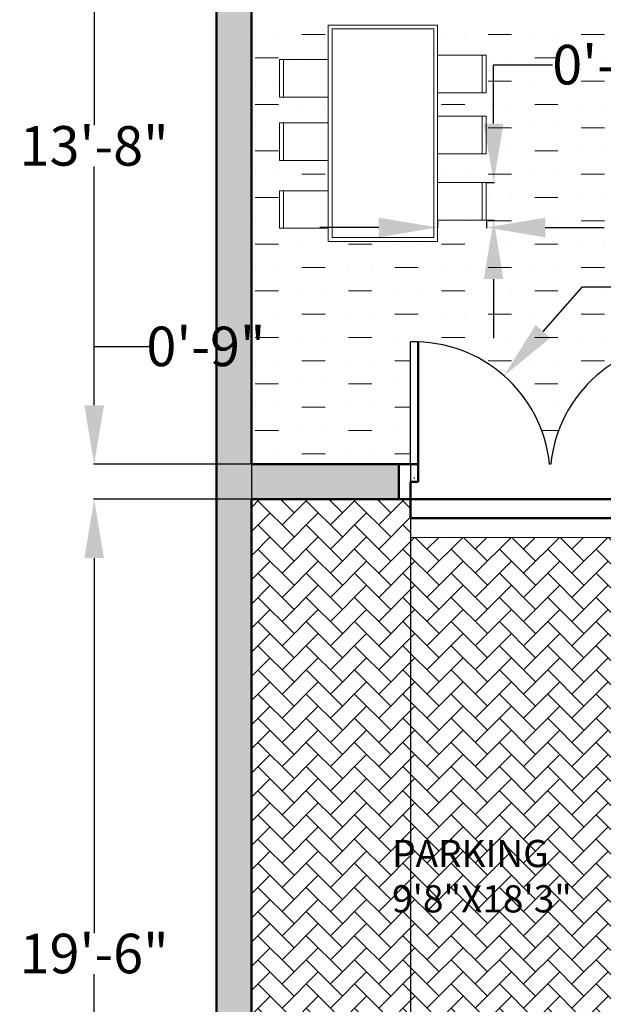
# Model space of a CAD drawing. Units: inches. Extents: x 26 to 14419, y 2 to 3479.
# Tile 2 of 9: x 13608 to 13759, y 2946 to 3199. Entities that reach past the tile are written whole.
import ezdxf

# ---------------------------------------------------------------- set-up
doc = ezdxf.new("R2010")
doc.units = ezdxf.units.IN
doc.header["$MEASUREMENT"] = 0
for name, color, linetype, lineweight in [('A-ANNO-DIMS', 2, 'Continuous', 18), ('A-AREA-IDEN', 7, 'Continuous', 18), ('A-DOOR', 4, 'Continuous', 25), ('A-FLOR-PATT', 252, 'Continuous', 13), ('A-FURN', 8, 'Continuous', 18), ('A-WALL', 7, 'Continuous', 50)]:
    doc.layers.add(name, color=color, linetype=linetype, lineweight=lineweight)
doc.styles.get("Standard").update_dxf_attribs({"font": 'arial.ttf'})
doc.dimstyles.get("Standard").update_dxf_attribs({"dimtxt": 10.18, "dimasz": 15.18, "dimexe": 0.18, "dimexo": 0.0625, "dimgap": 0.09, "dimtad": 0, "dimtih": 1, "dimtoh": 1, "dimdec": 0, "dimzin": 0, "dimdsep": 46, "dimlunit": 3, "dimtxsty": 'Standard', "dimcen": 0.09, "dimadec": 0, "dimazin": 0, "dimtfac": 1, "dimtdec": 0, "dimtofl": 0, "dimtmove": 0, "dimatfit": 3, "dimfxl": 1, "dimtolj": 1, "dimtzin": 0, "dimarcsym": 0})

# ---------------------------------------------------------------- blocks, each defined once
blk = doc.blocks.new('DOOR-DOUBLE')
for p, q in [((0, 0), (0, 31.5)), ((72, 0), (72, 31.5)), ((36.16, 0), (35.84, 0))]:
    blk.add_line(p, q)
for centre, start, end in [((1, -3.5), 5.7368, 91.6366), ((71, -3.5), 88.3634, 174.2632)]:
    blk.add_arc(centre, 35.01, start, end)
blk = doc.blocks.new('CHAIR')
blk.add_line((11.52, 9.68), (11.52, 0))
blk.add_lwpolyline([(0, 9.68), (12.56, 9.68), (12.56, 0), (0, 0)], close=True)
blk = doc.blocks.new('*D23')
at = {"layer": 'A-ANNO-DIMS', "color": 0, "lineweight": -2, "transparency": 16777216}
for p, q in [((13716.08, 3147.8), (13716.08, 3145.8)), ((13728.65, 3147.8), (13728.65, 3145.8)), ((13700.9, 3145.98), (13685.72, 3145.98)), ((13743.83, 3145.98), (13759.01, 3145.98))]:
    blk.add_line(p, q, dxfattribs=at)
at = {"layer": 'A-ANNO-DIMS', "color": 0, "transparency": 16777216}
for points in [[(13700.9, 3148.51), (13700.9, 3143.45), (13716.08, 3145.98)], [(13743.83, 3148.51), (13743.83, 3143.45), (13728.65, 3145.98)]]:
    blk.add_solid(points, dxfattribs=at)
at = {"layer": 'Defpoints', "color": 0, "transparency": 16777216}
for p in [(13716.08, 3147.87), (13728.65, 3147.87), (13728.65, 3145.98)]:
    blk.add_point(p, dxfattribs=at)
at = {"layer": 'A-ANNO-DIMS', "color": 0, "transparency": 16777216, "insert": (13826.02, 3145.98), "char_height": 10.18, "attachment_point": 5}
blk.add_mtext('\\A1;CHAIR 1\'-0 1/2" TYP.', dxfattribs=at)
blk = doc.blocks.new('*D24')
at = {"layer": 'A-ANNO-DIMS', "color": 0, "lineweight": -2, "transparency": 16777216}
for p, q in [((13730.53, 3172.73), (13730.53, 3187.91)), ((13730.53, 3187.91), (13745.71, 3187.91)), ((13728.71, 3157.55), (13730.71, 3157.55)), ((13728.71, 3147.87), (13730.71, 3147.87)), ((13730.53, 3132.69), (13730.53, 3117.51))]:
    blk.add_line(p, q, dxfattribs=at)
at = {"layer": 'A-ANNO-DIMS', "color": 0, "transparency": 16777216}
for points in [[(13728, 3172.73), (13733.06, 3172.73), (13730.53, 3157.55)], [(13728, 3132.69), (13733.06, 3132.69), (13730.53, 3147.87)]]:
    blk.add_solid(points, dxfattribs=at)
at = {"layer": 'Defpoints', "color": 0, "transparency": 16777216}
for p in [(13728.65, 3157.55), (13730.53, 3157.55), (13728.65, 3147.87)]:
    blk.add_point(p, dxfattribs=at)
at = {"layer": 'A-ANNO-DIMS', "color": 0, "transparency": 16777216, "insert": (13788.69, 3187.91), "char_height": 10.18, "attachment_point": 5}
blk.add_mtext('\\A1;0\'-9 1/2" TYP.', dxfattribs=at)
blk = doc.blocks.new('*D56')
at = {"layer": 'A-ANNO-DIMS', "color": 0, "lineweight": -2, "transparency": 16777216}
for p, q in [((13668.03, 3076), (13627.41, 3076)), ((13627.59, 3060.82), (13627.59, 2964.28)), ((13627.59, 2857.18), (13627.59, 2953.71)), ((13668.03, 2842), (13627.41, 2842))]:
    blk.add_line(p, q, dxfattribs=at)
at = {"layer": 'A-ANNO-DIMS', "color": 0, "transparency": 16777216}
for points in [[(13625.06, 3060.82), (13630.12, 3060.82), (13627.59, 3076)], [(13625.06, 2857.18), (13630.12, 2857.18), (13627.59, 2842)]]:
    blk.add_solid(points, dxfattribs=at)
at = {"layer": 'Defpoints', "color": 0, "transparency": 16777216}
for p in [(13627.59, 3076), (13668.09, 3076), (13668.09, 2842)]:
    blk.add_point(p, dxfattribs=at)
at = {"layer": 'A-ANNO-DIMS', "color": 0, "transparency": 16777216, "insert": (13627.59, 2959), "char_height": 10.18, "attachment_point": 5}
blk.add_mtext('\\A1;19\'-6"', dxfattribs=at)
blk = doc.blocks.new('*D57')
at = {"layer": 'A-ANNO-DIMS', "color": 0, "lineweight": -2, "transparency": 16777216}
for p, q in [((13627.59, 3100.18), (13627.59, 3115.36)), ((13627.59, 3115.36), (13642.77, 3115.36)), ((13668.03, 3085), (13627.41, 3085)), ((13668.03, 3076), (13627.41, 3076)), ((13627.59, 3060.82), (13627.59, 3045.64))]:
    blk.add_line(p, q, dxfattribs=at)
at = {"layer": 'A-ANNO-DIMS', "color": 0, "transparency": 16777216}
for points in [[(13625.06, 3100.18), (13630.12, 3100.18), (13627.59, 3085)], [(13625.06, 3060.82), (13630.12, 3060.82), (13627.59, 3076)]]:
    blk.add_solid(points, dxfattribs=at)
at = {"layer": 'Defpoints', "color": 0, "transparency": 16777216}
for p in [(13627.59, 3085), (13668.09, 3085), (13668.09, 3076)]:
    blk.add_point(p, dxfattribs=at)
at = {"layer": 'A-ANNO-DIMS', "color": 0, "transparency": 16777216, "insert": (13656.39, 3115.36), "char_height": 10.18, "attachment_point": 5}
blk.add_mtext('\\A1;0\'-9"', dxfattribs=at)
blk = doc.blocks.new('*D58')
at = {"layer": 'A-ANNO-DIMS', "color": 0, "lineweight": -2, "transparency": 16777216}
for p, q in [((13668.03, 3249), (13627.41, 3249)), ((13627.59, 3233.82), (13627.59, 3172.29)), ((13627.59, 3100.18), (13627.59, 3161.7)), ((13668.03, 3085), (13627.41, 3085))]:
    blk.add_line(p, q, dxfattribs=at)
at = {"layer": 'A-ANNO-DIMS', "color": 0, "transparency": 16777216}
for points in [[(13625.06, 3233.82), (13630.12, 3233.82), (13627.59, 3249)], [(13625.06, 3100.18), (13630.12, 3100.18), (13627.59, 3085)]]:
    blk.add_solid(points, dxfattribs=at)
at = {"layer": 'Defpoints', "color": 0, "transparency": 16777216}
for p in [(13627.59, 3249), (13668.09, 3249), (13668.09, 3085)]:
    blk.add_point(p, dxfattribs=at)
at = {"layer": 'A-ANNO-DIMS', "color": 0, "transparency": 16777216, "insert": (13627.59, 3167), "char_height": 10.18, "attachment_point": 5}
blk.add_mtext('\\A1;13\'-8"', dxfattribs=at)
blk = doc.blocks.new('*D73')
at = {"layer": 'A-ANNO-DIMS', "color": 0, "lineweight": -2, "transparency": 16777216}
for p, q in [((13668.09, 3084.93), (13668.09, 2810.32)), ((13709.09, 3084.93), (13709.09, 2810.32)), ((13683.27, 2810.5), (13693.91, 2810.5)), ((13709.09, 2810.5), (13724.27, 2810.5))]:
    blk.add_line(p, q, dxfattribs=at)
at = {"layer": 'A-ANNO-DIMS', "color": 0, "transparency": 16777216}
for points in [[(13683.27, 2813.03), (13683.27, 2807.97), (13668.09, 2810.5)], [(13693.91, 2813.03), (13693.91, 2807.97), (13709.09, 2810.5)]]:
    blk.add_solid(points, dxfattribs=at)
at = {"layer": 'Defpoints', "color": 0, "transparency": 16777216}
for p in [(13668.09, 3085), (13709.09, 3085), (13709.09, 2810.5)]:
    blk.add_point(p, dxfattribs=at)
at = {"layer": 'A-ANNO-DIMS', "color": 0, "transparency": 16777216, "insert": (13737.89, 2810.5), "char_height": 10.18, "attachment_point": 5}
blk.add_mtext('\\A1;3\'-5"', dxfattribs=at)
blk = doc.blocks.new('*D121')
at = {"layer": 'A-ANNO-DIMS', "color": 0, "lineweight": -2, "transparency": 16777216}
for p, q in [((13753.25, 3130.6), (13743.23, 3119.2)), ((13768.43, 3130.6), (13753.25, 3130.6)), ((13710, 3081.5), (13710.18, 3081.5)), ((13710.09, 3081.41), (13710.09, 3081.59))]:
    blk.add_line(p, q, dxfattribs=at)
at = {"layer": 'A-ANNO-DIMS', "color": 0, "transparency": 16777216}
blk.add_solid([(13741.33, 3120.87), (13745.13, 3117.53), (13733.21, 3107.8)], dxfattribs=at)
at = {"layer": 'Defpoints', "color": 0, "transparency": 16777216}
for p in [(13733.21, 3107.8), (13710.09, 3081.5)]:
    blk.add_point(p, dxfattribs=at)
at = {"layer": 'A-ANNO-DIMS', "color": 0, "transparency": 16777216, "insert": (13801.81, 3130.6), "char_height": 10.18, "attachment_point": 5}
blk.add_mtext('\\A1;5X R2\'-11"', dxfattribs=at)

msp = doc.modelspace()

# ---------------------------------------------------------------- hatches: boundary and pattern name
at = {"layer": 'A-FLOR-PATT'}
h = msp.add_hatch(color=256, dxfattribs=at)
h.dxf.hatch_style = 1
h.paths.add_polyline_path([(13922.09, 3432), (13659.09, 3432), (13659.09, 2842), (13668.09, 2842), (13668.09, 2851), (13668.09, 2899), (13668.09, 2908), (13668.09, 3076), (13706.09, 3076), (13706.09, 3085), (13668.09, 3085), (13668.09, 3249), (13712.76, 3249), (13712.76, 3255), (13668.09, 3255), (13668.09, 3375), (13720.94, 3375), (13720.94, 3378, -0.017236), (13720.94, 3380), (13720.94, 3381), (13668.09, 3381), (13668.09, 3423), (13784.09, 3423), (13784.09, 3381), (13753.94, 3381), (13753.94, 3375), (13784.09, 3375), (13784.09, 3255), (13758.77, 3255), (13758.77, 3249), (13784.09, 3249), (13793.09, 3249), (13793.09, 3255), (13793.09, 3423), (13913.09, 3423), (13913.09, 3255), (13832.09, 3255), (13832.09, 3254, -0.014283), (13832.09, 3252), (13832.09, 3249), (13836.57, 3249), (13836.57, 3234), (13839.57, 3234, -0.017236), (13841.57, 3234), (13842.57, 3234), (13842.57, 3249), (13913.09, 3249), (13913.09, 3201), (13892.46, 3201), (13793.09, 3201), (13784.09, 3201), (13784.09, 3195), (13793.09, 3195), (13913.09, 3195), (13913.09, 3127), (13922.09, 3127)])
h.paths.add_polyline_path([(13922.09, 3013.5), (13913.09, 3013.5), (13913.09, 2908), (13892.09, 2908), (13892.09, 2899), (13913.09, 2899), (13913.09, 2851), (13793.09, 2851), (13784.09, 2851), (13784.09, 2842), (13922.09, 2842)], flags=17)
h.paths.add_polyline_path([(13793.09, 3085), (13784.09, 3085), (13784.09, 3076), (13784.09, 3071.08), (13784.09, 3066.17), (13784.09, 2908), (13784.09, 2899.07), (13793.09, 2899), (13802.09, 2899), (13814.09, 2899), (13814.09, 2908), (13793.09, 2908)], flags=17)
h.paths.add_polyline_path([(14342.64, 3401.72), (14242.78, 3401.72), (14242.78, 3392.72), (14257.64, 3392.72), (14257.64, 3351.75), (14257.64, 3345.75), (14257.64, 3330.73), (14263.64, 3330.73), (14263.64, 3392.72), (14333.64, 3392.72), (14333.64, 3284.72), (14302.92, 3284.72), (14302.92, 3281.72, -0.022645), (14302.92, 3279.12), (14302.92, 3278.72), (14333.64, 3278.72), (14333.64, 3170.72), (14316.1, 3170.72), (14263.64, 3170.72), (14263.64, 3278.72), (14269.92, 3278.72), (14269.92, 3284.72), (14263.64, 3284.72), (14257.64, 3284.72), (14257.64, 3225.75), (14257.64, 3219.75), (14257.64, 3164.72), (14333.64, 3164.72), (14333.64, 3110.37), (14210.01, 3110.37), (14210.01, 3104.37), (14257.64, 3104.37), (14257.64, 3024), (14263.64, 3024), (14263.64, 3039.72), (14263.64, 3104.37), (14333.64, 3104.37), (14333.64, 3045.72), (14333.64, 3039.72), (14333.64, 2967.72), (14296.64, 2967.72), (14296.64, 2964.72, -0.017236), (14296.64, 2962.72), (14296.64, 2961.72), (14333.64, 2961.72), (14333.64, 2882.72), (14312.64, 2882.72), (14312.64, 2873.72), (14333.64, 2873.72), (14333.64, 2820.72), (14333.64, 2811.72), (14342.64, 2811.72)])
h.paths.add_polyline_path([(14088.64, 3219.75), (14218.64, 3219.75), (14218.64, 3222.75, -0.014283), (14218.64, 3224.75), (14218.64, 3225.75), (14088.64, 3225.75), (14088.64, 3345.75), (14088.64, 3351.75), (14088.64, 3392.72), (14193.93, 3392.72), (14193.93, 3351.75), (14140.64, 3351.75), (14140.64, 3345.75), (14170.7, 3345.75), (14218.64, 3345.75), (14218.64, 3348.75, -0.014283), (14218.64, 3350.75), (14218.64, 3351.75), (14199.93, 3351.75), (14199.93, 3392.72), (14214.78, 3392.72), (14214.78, 3401.72), (14079.64, 3401.72), (14079.64, 2811.72), (14088.64, 2811.72), (14088.64, 2820.72), (14088.64, 2873.72), (14116.21, 2873.72), (14116.21, 2876.57), (14116.21, 2882.72), (14088.64, 2882.72), (14088.64, 3039.72), (14216.01, 3039.72), (14216.01, 3065.37), (14215.01, 3065.37, -0.014283), (14213.01, 3065.37), (14210.01, 3065.37), (14210.01, 3045.72), (14154.64, 3045.72), (14148.64, 3045.72), (14088.64, 3045.72)])
h.paths.add_polyline_path([(14284.64, 2882.72), (14263.64, 2882.72), (14263.64, 2961.72), (14263.64, 2967.72), (14257.64, 2967.72), (14257.64, 2956.69), (14257.64, 2916.18), (14257.64, 2882.72), (14249.61, 2882.72), (14249.61, 2873.72), (14284.64, 2873.72)], flags=17)
h.paths.add_polyline_path([(14202.78, 2882.72), (14189.55, 2882.72), (14189.55, 2879.95), (14189.55, 2873.72), (14202.78, 2873.72)], flags=17)
h = msp.add_hatch(dxfattribs=at)
h.set_pattern_fill('MUDST', color=256, scale=24)
h.set_pattern_definition([(0, (61.093, 57.669), (12, 6), [6, -6, 0, -6, 0, -6])])
h.paths.add_polyline_path([(13756.28, 3375), (13750.94, 3375), (13720.94, 3375), (13706.54, 3375), (13706.54, 3255), (13712.76, 3255), (13712.76, 3249), (13668.09, 3249), (13668.09, 3085), (13709.09, 3085), (13709.09, 3116.5, -0.393405), (13744.93, 3085), (13745.25, 3085, -0.393405), (13781.09, 3116.5), (13781.09, 3085), (13784.09, 3085), (13784.09, 3127), (13784.09, 3195), (13784.09, 3201), (13793.09, 3201), (13836.57, 3201), (13836.57, 3204), (13836.57, 3234), (13836.57, 3249), (13832.09, 3249), (13832.09, 3254, 0.397579), (13798.09, 3288), (13798.09, 3252), (13796.09, 3252), (13796.09, 3249), (13793.09, 3249), (13784.09, 3249), (13758.77, 3249), (13758.77, 3255), (13784.09, 3255), (13784.09, 3303.43), (13756.28, 3303.43)])
h.paths.add_polyline_path([(13757.29, 3298.63), (13757.76, 3298.12), (13779.63, 3298.12), (13779.63, 3268.87), (13757.77, 3268.87), (13756.19, 3268.87), (13756.19, 3285.02), (13757.77, 3285.02), (13757.77, 3298.11), (13749.96, 3290.89), (13749.48, 3291.4)], flags=16)
h.paths.add_polyline_path([(13758.77, 3297.12), (13778.63, 3297.12), (13778.63, 3269.87), (13758.77, 3269.87)], flags=0)
h.paths.add_polyline_path([(13716.08, 3198.11), (13716.08, 3190.37), (13728.65, 3190.37), (13728.65, 3180.68), (13716.08, 3180.68), (13716.08, 3174.63), (13728.65, 3174.63), (13728.65, 3164.95), (13716.08, 3164.95), (13716.08, 3157.55), (13728.65, 3157.55), (13728.65, 3147.87), (13716.08, 3147.87), (13716.08, 3142.39), (13687.89, 3142.39), (13687.89, 3145.78), (13675.33, 3145.78), (13675.33, 3155.46), (13687.89, 3155.46), (13687.89, 3163.27), (13675.33, 3163.27), (13675.33, 3172.95), (13687.89, 3172.95), (13687.89, 3179.58), (13675.33, 3179.58), (13675.33, 3189.26), (13687.89, 3189.26), (13687.89, 3198.11)], flags=16)
h.paths.add_polyline_path([(13715.08, 3197.11), (13715.08, 3143.39), (13688.89, 3143.39), (13688.89, 3197.11)], flags=0)
h = msp.add_hatch(dxfattribs=at)
h.set_pattern_fill('AR-HBONE', color=256, scale=1.1)
h.set_pattern_definition([(45, (61.093, 57.669), (0, 6.2225397), [13.2, -4.4]), (135, (64.2045, 60.7802), (5e-16, 6.2225397), [13.2, -4.4])])
h.paths.add_polyline_path([(13668.09, 2908), (13668.09, 2899), (13668.09, 2851), (13668.09, 2842), (13784.09, 2842), (13784.09, 2851), (13784.09, 2899), (13784.09, 2908), (13784.09, 3066.17), (13709.09, 3066.17), (13709.09, 3071.08), (13709.09, 3076), (13668.09, 3076)])

# ---------------------------------------------------------------- linework, layer by layer
at = {"layer": 'A-FURN'}
for points in [[(13687.89, 3198.11), (13716.08, 3198.11), (13716.08, 3142.39), (13687.89, 3142.39)], [(13688.89, 3197.11), (13715.08, 3197.11), (13715.08, 3143.39), (13688.89, 3143.39)], [(13709.09, 3071.08), (13784.09, 3071.08), (13784.09, 3066.17), (13709.09, 3066.17)]]:
    msp.add_lwpolyline(points, close=True, dxfattribs=at)
at = {"layer": 'A-WALL'}
for p, q in [((13659.09, 2842), (13659.09, 3432)), ((13668.09, 3085), (13668.09, 3249)), ((13711.09, 3080.5), (13711.09, 3116.5)), ((13711.09, 3085), (13668.09, 3085)), ((13706.09, 3085), (13706.09, 3076)), ((13709.09, 3080.5), (13709.09, 3076)), ((13711.09, 3080.5), (13709.09, 3080.5)), ((13668.09, 2908), (13668.09, 3076)), ((13709.09, 3076), (13668.09, 3076))]:
    msp.add_line(p, q, dxfattribs=at)
msp.add_lwpolyline([(13709.09, 3076), (13784.09, 3076), (13784.09, 3071.08), (13709.09, 3071.08)], close=True, dxfattribs=at)

# ---------------------------------------------------------------- block references
at = {"layer": 'A-DOOR'}
msp.add_blockref('DOOR-DOUBLE', (13709.09, 3085), dxfattribs=at)
at = {"layer": 'A-FURN'}
for p in [(13716.08, 3180.68), (13716.08, 3164.95), (13716.08, 3147.87)]:
    msp.add_blockref('CHAIR', p, dxfattribs=at)
at = {"layer": 'A-FURN', "rotation": 180}
for p in [(13687.89, 3189.26), (13687.89, 3172.95), (13687.89, 3155.46)]:
    msp.add_blockref('CHAIR', p, dxfattribs=at)

# ---------------------------------------------------------------- texts
at = {"layer": 'A-AREA-IDEN', "insert": (13704.35, 2988.26), "char_height": 7, "attachment_point": 1}
msp.add_mtext_dynamic_manual_height_columns('PARKING\\P9\'8"X18\'3"', width=51, gutter_width=1, heights=[0], dxfattribs=at)

# ---------------------------------------------------------------- dimensions: what is measured, and where the dimension line sits
at = {"layer": 'A-ANNO-DIMS'}
for base, p1, p2, picture, middle in [((13627.59, 3249), (13668.09, 3085), (13668.09, 3249), '*D58', (13627.59, 3167)), ((13627.59, 3085), (13668.09, 3076), (13668.09, 3085), '*D57', (13656.39, 3115.36)), ((13627.59, 3076), (13668.09, 2842), (13668.09, 3076), '*D56', (13627.59, 2959))]:
    dim = msp.add_linear_dim(base=base, p1=p1, p2=p2, angle=90, dimstyle='Standard', override={"dimdec": 1, "dimlfac": 1, "dimrnd": 0, "dimzin": 1, "dimdsep": 46, "dimlunit": 4, "dimfrac": 2}, dxfattribs=at)
    dim.commit()
    dim.dimension.update_dxf_attribs({"geometry": picture, "text_midpoint": middle})
dim = msp.add_linear_dim(base=(13730.53, 3157.55), p1=(13728.65, 3147.87), p2=(13728.65, 3157.55), angle=90, text='<> TYP.', dimstyle='Standard', override={"dimdec": 1, "dimrnd": 0, "dimzin": 1, "dimlunit": 4, "dimfrac": 2}, dxfattribs=at)
dim.commit()
dim.dimension.update_dxf_attribs({"geometry": '*D24', "text_midpoint": (13788.69, 3187.91)})
dim = msp.add_linear_dim(base=(13728.65, 3145.98), p1=(13716.08, 3147.87), p2=(13728.65, 3147.87), text='CHAIR <> TYP.', dimstyle='Standard', override={"dimdec": 1, "dimrnd": 0, "dimzin": 1, "dimlunit": 4, "dimfrac": 2}, dxfattribs=at)
dim.commit()
dim.dimension.update_dxf_attribs({"geometry": '*D23', "text_midpoint": (13826.02, 3145.98)})
dim = msp.add_radius_dim(center=(13710.09, 3081.5), mpoint=(13733.21, 3107.8), text='5X <>', dimstyle='Standard', override={"dimdec": 1, "dimlfac": 1, "dimrnd": 0, "dimzin": 1, "dimdsep": 46, "dimlunit": 4, "dimfrac": 2}, dxfattribs=at)
dim.commit()
dim.dimension.update_dxf_attribs({"geometry": '*D121', "text_midpoint": (13801.81, 3130.6)})
dim = msp.add_linear_dim(base=(13709.09, 2810.5), p1=(13668.09, 3085), p2=(13709.09, 3085), dimstyle='Standard', override={"dimdec": 1, "dimlfac": 1, "dimrnd": 0, "dimzin": 1, "dimdsep": 46, "dimlunit": 4, "dimfrac": 2}, dxfattribs=at)
dim.commit()
dim.dimension.update_dxf_attribs({"geometry": '*D73', "text_midpoint": (13737.89, 2810.5)})

doc.saveas('drawing.dxf')
